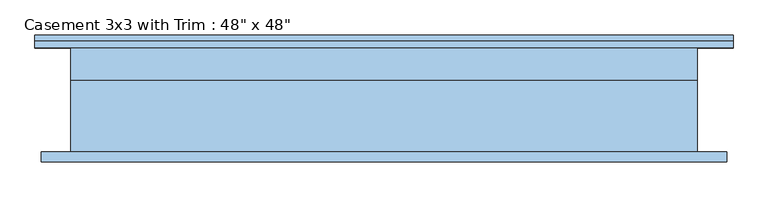
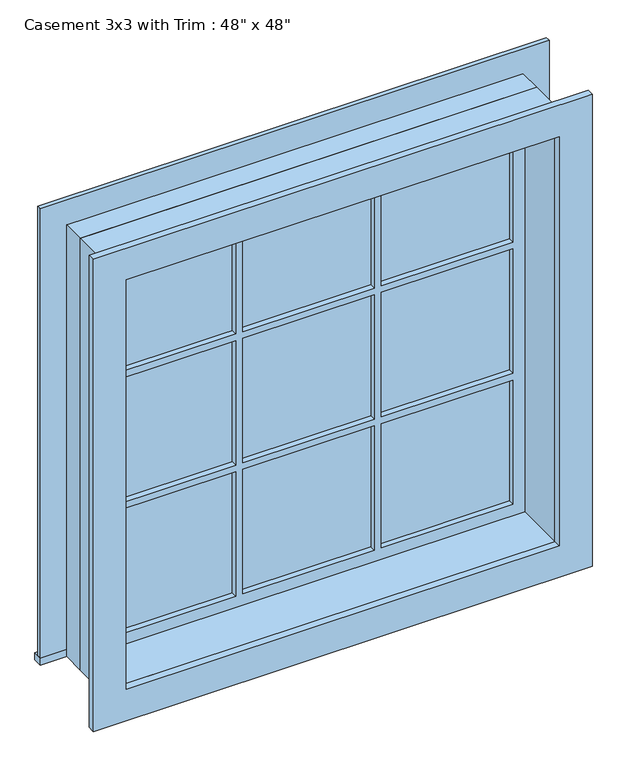
"""IFC4 building model written with IfcOpenShell, lengths in millimetres: window geometry."""

from ifc_helpers import new_model, si_unit, frame, origin, place, context, project, spatial, polyline, outline, extrude, source, transform, mapped, element, save


def window_3ea3e93d(model_context):
    return source(origin(), model_context, "Body", "SweptSolid", [
        extrude(outline(polyline([(-679.45, 127.0), (679.45, 127.0), (679.45, 101.6), (-679.45, 101.6), (-679.45, 127.0)])), frame((0.0, 0.0, 609.6), z_axis=(0.0, 0.0, 1.0), x_axis=(1.0, 0.0, 0.0)), (0.0, 0.0, 1.0), 19.05),
        extrude(outline(polyline([(1809.75, -590.55), (1809.75, 590.55), (628.65, 590.55), (628.65, 679.45), (1898.65, 679.45), (1898.65, -679.45), (628.65, -679.45), (628.65, -590.55), (1809.75, -590.55)])), frame((0.0, 101.6, 0.0), z_axis=(0.0, 1.0, 0.0), x_axis=(0.0, 0.0, 1.0)), (0.0, 0.0, 1.0), 12.7),
        extrude(outline(polyline([(194.7333333, 66.675), (546.1, 66.675), (546.1, 53.975), (194.7333333, 53.975), (194.7333333, 66.675)])), frame((0.0, 0.0, 1413.9333333), z_axis=(0.0, 0.0, 1.0), x_axis=(1.0, 0.0, 0.0)), (0.0, 0.0, 1.0), 351.3666667),
        extrude(outline(polyline([(-175.6833333, 66.675), (175.6833333, 66.675), (175.6833333, 53.975), (-175.6833333, 53.975), (-175.6833333, 66.675)])), frame((0.0, 0.0, 1413.9333333), z_axis=(0.0, 0.0, 1.0), x_axis=(1.0, 0.0, 0.0)), (0.0, 0.0, 1.0), 351.3666667),
        extrude(outline(polyline([(-546.1, 66.675), (-194.7333333, 66.675), (-194.7333333, 53.975), (-546.1, 53.975), (-546.1, 66.675)])), frame((0.0, 0.0, 1413.9333333), z_axis=(0.0, 0.0, 1.0), x_axis=(1.0, 0.0, 0.0)), (0.0, 0.0, 1.0), 351.3666667),
        extrude(outline(polyline([(-546.1, 66.675), (-194.7333333, 66.675), (-194.7333333, 53.975), (-546.1, 53.975), (-546.1, 66.675)])), frame((0.0, 0.0, 1043.5166667), z_axis=(0.0, 0.0, 1.0), x_axis=(1.0, 0.0, 0.0)), (0.0, 0.0, 1.0), 351.3666667),
        extrude(outline(polyline([(-175.6833333, 66.675), (175.6833333, 66.675), (175.6833333, 53.975), (-175.6833333, 53.975), (-175.6833333, 66.675)])), frame((0.0, 0.0, 1043.5166667), z_axis=(0.0, 0.0, 1.0), x_axis=(1.0, 0.0, 0.0)), (0.0, 0.0, 1.0), 351.3666667),
        extrude(outline(polyline([(194.7333333, 66.675), (546.1, 66.675), (546.1, 53.975), (194.7333333, 53.975), (194.7333333, 66.675)])), frame((0.0, 0.0, 1043.5166667), z_axis=(0.0, 0.0, 1.0), x_axis=(1.0, 0.0, 0.0)), (0.0, 0.0, 1.0), 351.3666667),
        extrude(outline(polyline([(194.7333333, 66.675), (546.1, 66.675), (546.1, 53.975), (194.7333333, 53.975), (194.7333333, 66.675)])), frame((0.0, 0.0, 673.1), z_axis=(0.0, 0.0, 1.0), x_axis=(1.0, 0.0, 0.0)), (0.0, 0.0, 1.0), 351.3666667),
        extrude(outline(polyline([(-175.6833333, 66.675), (175.6833333, 66.675), (175.6833333, 53.975), (-175.6833333, 53.975), (-175.6833333, 66.675)])), frame((0.0, 0.0, 673.1), z_axis=(0.0, 0.0, 1.0), x_axis=(1.0, 0.0, 0.0)), (0.0, 0.0, 1.0), 351.3666667),
        extrude(outline(polyline([(-546.1, 66.675), (-194.7333333, 66.675), (-194.7333333, 53.975), (-546.1, 53.975), (-546.1, 66.675)])), frame((0.0, 0.0, 673.1), z_axis=(0.0, 0.0, 1.0), x_axis=(1.0, 0.0, 0.0)), (0.0, 0.0, 1.0), 351.3666667),
        extrude(outline(polyline([(1885.95, 666.75), (1885.95, -666.75), (552.45, -666.75), (552.45, 666.75), (1885.95, 666.75)]), holes=[polyline([(1797.05, 577.85), (641.35, 577.85), (641.35, -577.85), (1797.05, -577.85), (1797.05, 577.85)])]), frame((0.0, -120.65, 0.0), z_axis=(0.0, 1.0, 0.0), x_axis=(0.0, 0.0, 1.0)), (0.0, 0.0, 1.0), 19.05),
        extrude(outline(polyline([(1809.75, -590.55), (628.65, -590.55), (628.65, 590.55), (1809.75, 590.55), (1809.75, -590.55)]), holes=[polyline([(1765.3, -194.7333333), (1413.9333333, -194.7333333), (1413.9333333, -546.1), (1765.3, -546.1), (1765.3, -194.7333333)]), polyline([(1394.8833333, -194.7333333), (1043.5166667, -194.7333333), (1043.5166667, -546.1), (1394.8833333, -546.1), (1394.8833333, -194.7333333)]), polyline([(1024.4666667, -194.7333333), (673.1, -194.7333333), (673.1, -546.1), (1024.4666667, -546.1), (1024.4666667, -194.7333333)]), polyline([(1765.3, 175.6833333), (1413.9333333, 175.6833333), (1413.9333333, -175.6833333), (1765.3, -175.6833333), (1765.3, 175.6833333)]), polyline([(1394.8833333, 175.6833333), (1043.5166667, 175.6833333), (1043.5166667, -175.6833333), (1394.8833333, -175.6833333), (1394.8833333, 175.6833333)]), polyline([(1024.4666667, 175.6833333), (673.1, 175.6833333), (673.1, -175.6833333), (1024.4666667, -175.6833333), (1024.4666667, 175.6833333)]), polyline([(1765.3, 546.1), (1413.9333333, 546.1), (1413.9333333, 194.7333333), (1765.3, 194.7333333), (1765.3, 546.1)]), polyline([(1394.8833333, 546.1), (1043.5166667, 546.1), (1043.5166667, 194.7333333), (1394.8833333, 194.7333333), (1394.8833333, 546.1)]), polyline([(1024.4666667, 546.1), (673.1, 546.1), (673.1, 194.7333333), (1024.4666667, 194.7333333), (1024.4666667, 546.1)])]), frame((0.0, 38.1, 0.0), z_axis=(0.0, 1.0, 0.0), x_axis=(0.0, 0.0, 1.0)), (0.0, 0.0, 1.0), 44.45),
        extrude(outline(polyline([(1828.8, -609.6), (609.6, -609.6), (609.6, 609.6), (1828.8, 609.6), (1828.8, -609.6)]), holes=[polyline([(1797.05, -577.85), (1797.05, 577.85), (641.35, 577.85), (641.35, -577.85), (1797.05, -577.85)])]), frame((0.0, -101.6, 0.0), z_axis=(0.0, 1.0, 0.0), x_axis=(0.0, 0.0, 1.0)), (0.0, 0.0, 1.0), 139.7),
        extrude(outline(polyline([(1828.8, 609.6), (1828.8, -609.6), (609.6, -609.6), (609.6, 609.6), (1828.8, 609.6)]), holes=[polyline([(1809.75, 590.55), (628.65, 590.55), (628.65, -590.55), (1809.75, -590.55), (1809.75, 590.55)])]), frame((0.0, 38.1, 0.0), z_axis=(0.0, 1.0, 0.0), x_axis=(0.0, 0.0, 1.0)), (0.0, 0.0, 1.0), 63.5),
    ])


if __name__ == "__main__":
    model = new_model("IFC4")
    model_context = context("Model", 3, world=origin())
    ifc_project = project(units=[si_unit("LENGTHUNIT", "METRE", prefix="MILLI")], contexts=[model_context])
    site = spatial("IfcSite", under=ifc_project)
    building = spatial("IfcBuilding", under=site)
    placement = place(None, origin())
    window_shape = window_3ea3e93d(model_context)
    element("IfcWindow", 1, ObjectType="Casement 3x3 with Trim : 48\" x 48\"", at=placement, inside=building, context=model_context, shape_type="MappedRepresentation", body=[
        mapped(window_shape, transform((0.0, 0.0, 0.0), x_axis=(1.0, 0.0, 0.0), y_axis=(0.0, 1.0, 0.0), z_axis=(0.0, 0.0, 1.0))),
    ])
    save(model, "model.ifc")

# Revit data of these elements
# Type "Casement 3x3 with Trim : 48\" x 48\""
#   Type Mark = "11"
#   Construction Type Id = "GSP4R"
#   Assembly Code = "B2020100"
#   Analytic Construction = "1/8 in Pilkington single glazing"
#   Visual Light Transmittance = 0.9
#   Solar Heat Gain Coefficient = 0.78
#   Heat Transfer Coefficient (U) = 0.6496 BTU/(h·ft²·°F)
#   Height = 4' - 0"
#   Default Sill Height = 2' - 0"
#   Trim Projection - Ext. = 0' - 0 1/2"
#   Trim Projection - Int. = 0' - 0 3/4"
#   Trim Width - Exterior = 0' - 3 1/2"
#   Trim Width - Interior = 0' - 3 1/2"
#   Width = 4' - 0"
#   Window Inset = 0' - 0 3/4"
#   Define Thermal Properties by = 1
#   Glass Pane Material = Glass
#   Sash Material = Sash
#   Trim Exterior Material = Trim
#   Trim Interior Material = Trim
#   Wall Closure = (empty or 0)
# Element 1 (IfcWindow, "Casement 3x3 with Trim : 48\" x 48\"")
#   Materials on its faces: "Sash", "Glass", "Trim"
# Materials
#   "Glass": class "Glass", colour RGB 0 128 192, transparency 0.75, Description = "Soda Lime Glass", Cost = 0
#   "Sash": class "Wood", colour RGB 224 178 126, transparency 0
#   "Trim": class "Wood", colour RGB 224 178 126, transparency 0
